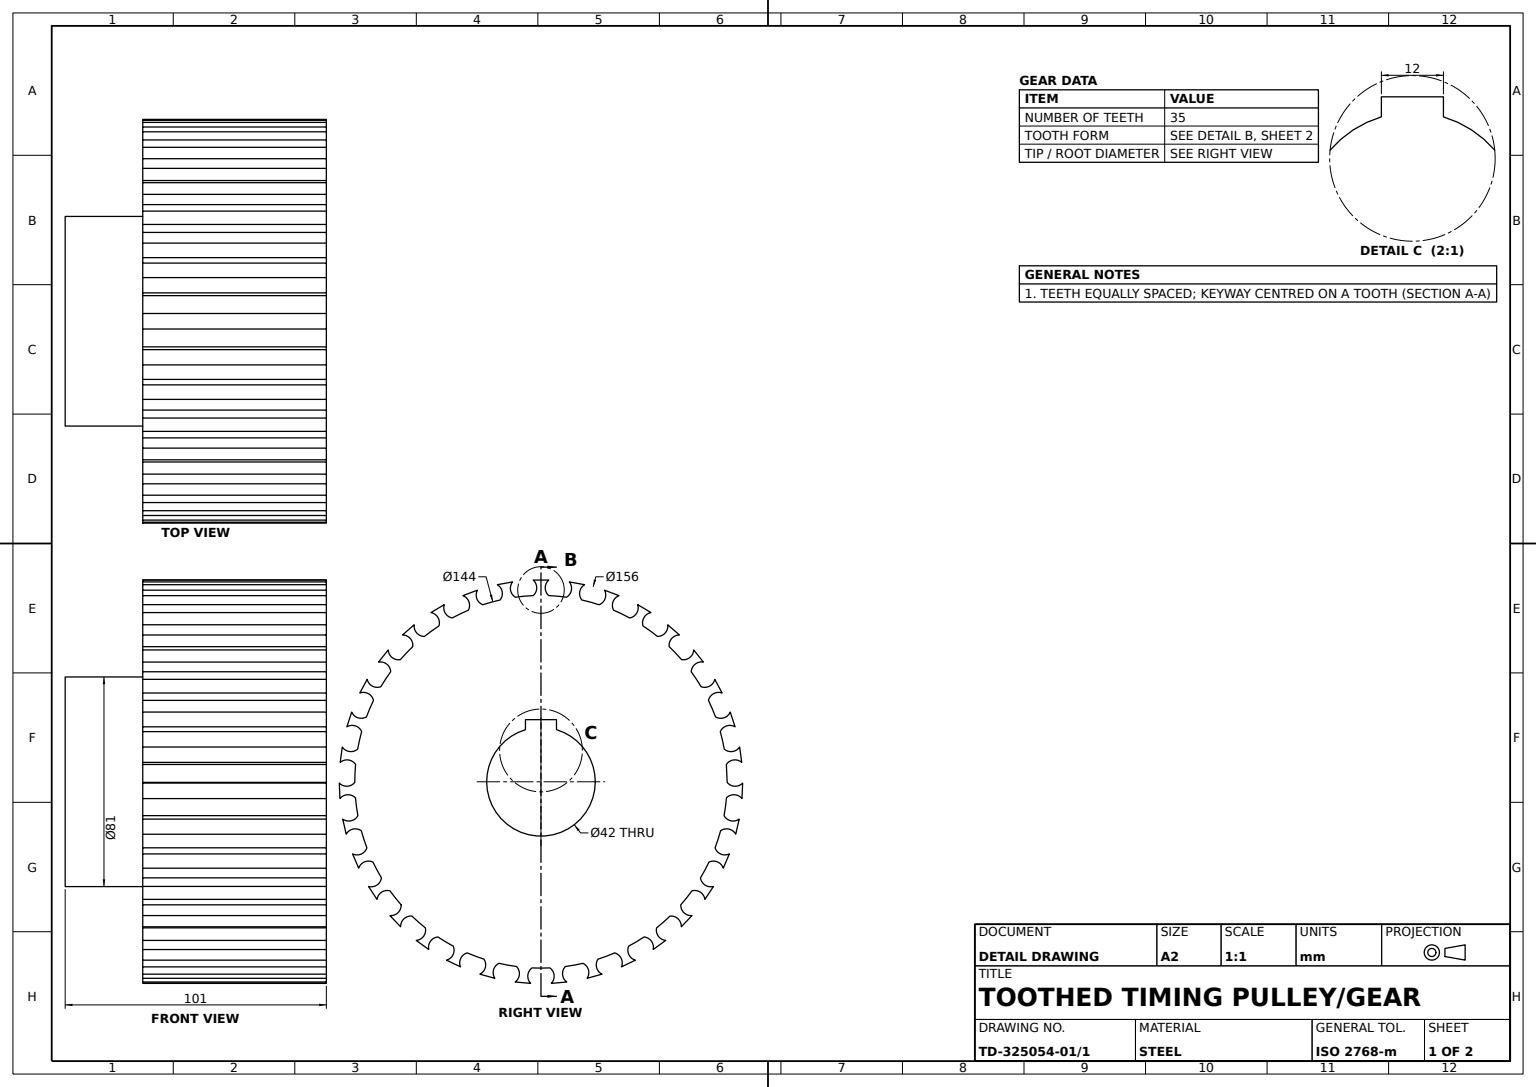
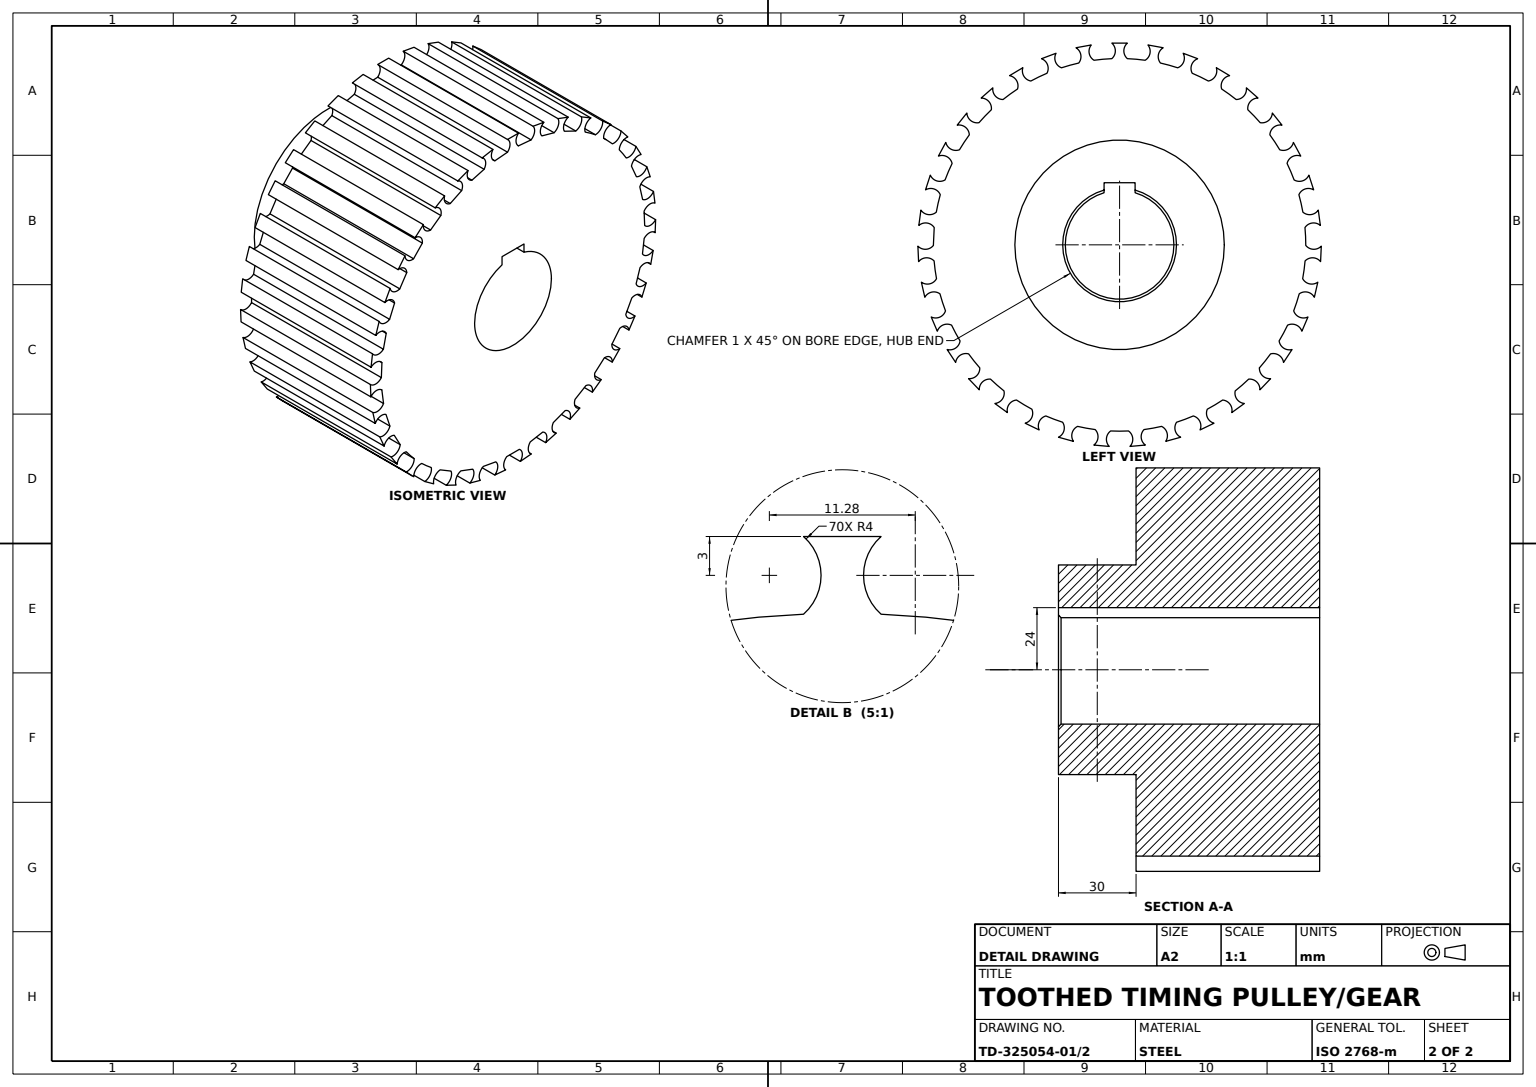
from build123d import *

# Parameters (mm, degrees)
GEAR_BODY_35T_DEPTH       = 71
HUB_SKETCH_R              = 40.5
HUB_81_DEPTH              = 30
BORE_42_WITH_KEYWAY_DEPTH = 150.561858306
EDGE_CHAMFER_1X45_SIZE    = 1


with BuildPart() as part:
    # Gear Tooth Profile Sketch → Gear Body 35T (new body)
    with BuildSketch(Plane.XY):
        with BuildLine():
            ThreePointArc((2.999348888, 77.942311399), (0, 78), (-2.999348888, 77.942311399))
            ThreePointArc((-2.999348888, 77.942311399), (-1.642369889, 74.9399057), (-2.999348888, 71.9375))
            ThreePointArc((-2.999348888, 71.9375), (-6.454030241, 71.710149168), (-9.893788502, 71.316989204))
            ThreePointArc((-9.893788502, 71.316989204), (-11.765060529, 74.028847052), (-10.96598898, 77.225300813))
            ThreePointArc((-10.96598898, 77.225300813), (-13.927437794, 76.746507911), (-16.868285214, 76.154191966))
            ThreePointArc((-16.868285214, 76.154191966), (-14.997013188, 73.442334117), (-15.796084737, 70.245880356))
            ThreePointArc((-15.796084737, 70.245880356), (-19.154652881, 69.40532597), (-22.468931389, 68.404291694))
            ThreePointArc((-22.468931389, 68.404291694), (-24.794352221, 70.738440349), (-24.578870939, 74.026205518))
            ThreePointArc((-24.578870939, 74.026205518), (-27.407236278, 73.02631991), (-30.195060974, 71.918414142))
            ThreePointArc((-30.195060974, 71.918414142), (-27.869640143, 69.584265487), (-28.085121425, 66.296500319))
            ThreePointArc((-28.085121425, 66.296500319), (-31.239629216, 64.869758489), (-34.321904334, 63.293023967))
            ThreePointArc((-34.321904334, 63.293023967), (-37.026733032, 65.17444197), (-37.401767762, 68.447847068))
            ThreePointArc((-37.401767762, 68.447847068), (-40.006143638, 66.959005901), (-42.55134263, 65.371119314))
            ThreePointArc((-42.55134263, 65.371119314), (-39.846513932, 63.489701311), (-39.471479203, 60.216296213))
            ThreePointArc((-39.471479203, 60.216296213), (-42.320538165, 58.249223595), (-45.071743033, 56.147466371))
            ThreePointArc((-45.071743033, 56.147466371), (-48.069044178, 57.5156834), (-49.022540995, 60.669518495))
            ThreePointArc((-49.022540995, 60.669518495), (-51.319220623, 58.739574348), (-53.539989123, 56.722742923))
            ThreePointArc((-53.539989123, 56.722742923), (-50.542687978, 55.354525895), (-49.589191161, 52.2006908))
            ThreePointArc((-49.589191161, 52.2006908), (-52.041230196, 49.756510727), (-54.372938826, 47.197283009))
            ThreePointArc((-54.372938826, 47.197283009), (-57.566376692, 48.008323441), (-59.067689425, 50.941221678))
            ThreePointArc((-59.067689425, 50.941221678), (-60.982855633, 48.632204545), (-62.807816312, 46.251250903))
            ThreePointArc((-62.807816312, 46.251250903), (-59.614378446, 45.440210471), (-58.113065714, 42.507312234))
            ThreePointArc((-58.113065714, 42.507312234), (-60.089274268, 39.664582665), (-61.926543627, 36.730140136))
            ThreePointArc((-61.926543627, 36.730140136), (-65.213478494, 36.957936466), (-67.214353715, 39.575632082))
            ThreePointArc((-67.214353715, 39.575632082), (-68.686451485, 36.961755673), (-70.056948606, 34.293205624))
            ThreePointArc((-70.056948606, 34.293205624), (-66.77001374, 34.065409294), (-64.769138519, 31.447713678))
            ThreePointArc((-64.769138519, 31.447713678), (-66.205999624, 28.297802279), (-67.489778363, 25.082460337))
            ThreePointArc((-67.489778363, 25.082460337), (-70.764565439, 24.719691003), (-73.200693373, 26.938049107))
            ThreePointArc((-73.200693373, 26.938049107), (-74.182408271, 24.103325561), (-75.05439293, 21.232948499))
            ThreePointArc((-75.05439293, 21.232948499), (-71.779605853, 21.595717833), (-69.343477919, 19.377359729))
            ThreePointArc((-69.343477919, 19.377359729), (-70.194809677, 16.021507245), (-70.883836091, 12.628609625))
            ThreePointArc((-70.883836091, 12.628609625), (-74.041221026, 11.686934333), (-76.834302516, 13.43465507))
            ThreePointArc((-76.834302516, 13.43465507), (-77.294081418, 10.470194734), (-77.639527309, 7.490246939))
            ThreePointArc((-77.639527309, 7.490246939), (-74.482142374, 8.431922232), (-71.689060884, 6.684201494))
            ThreePointArc((-71.689060884, 6.684201494), (-71.927500791, 3.230267785), (-71.999629003, -0.23113499))
            ThreePointArc((-71.999629003, -0.23113499), (-74.938130848, -1.721450024), (-77.998393957, -0.500539835))
            ThreePointArc((-77.998393957, -0.500539835), (-77.92145919, -3.499456767), (-77.729263399, -6.493197321))
            ThreePointArc((-77.729263399, -6.493197321), (-74.790761555, -5.002882288), (-71.730498445, -6.223792476))
            ThreePointArc((-71.730498445, -6.223792476), (-71.348382847, -9.664795139), (-70.801294598, -13.083450738))
            ThreePointArc((-70.801294598, -13.083450738), (-73.426467484, -15.07450556), (-76.655552839, -14.419646978))
            ThreePointArc((-76.655552839, -14.419646978), (-76.04437715, -17.356632849), (-75.320717007, -20.267944876))
            ThreePointArc((-75.320717007, -20.267944876), (-72.695544121, -18.276890054), (-69.466458767, -18.931748635))
            ThreePointArc((-69.466458767, -18.931748635), (-68.476069173, -22.249223595), (-67.327348329, -25.515253613))
            ThreePointArc((-67.327348329, -25.515253613), (-69.554817041, -27.943054084), (-72.84893918, -27.875294803))
            ThreePointArc((-72.84893918, -27.875294803), (-71.723166259, -30.655952469), (-70.491300797, -33.391264007))
            ThreePointArc((-70.491300797, -33.391264007), (-68.263832085, -30.963463536), (-64.969709946, -31.031222816))
            ThreePointArc((-64.969709946, -31.031222816), (-63.402878294, -34.118543698), (-61.689445688, -37.126975243))
            ThreePointArc((-61.689445688, -37.126975243), (-63.447617548, -39.913489858), (-66.700900676, -40.435007717))
            ThreePointArc((-66.700900676, -40.435007717), (-65.09671379, -42.969964553), (-63.396236178, -45.441360437))
            ThreePointArc((-63.396236178, -45.441360437), (-61.638064319, -42.654845823), (-58.384781191, -42.133327963))
            ThreePointArc((-58.384781191, -42.133327963), (-56.291866738, -44.891265734), (-54.068793504, -47.545405341))
            ThreePointArc((-54.068793504, -47.545405341), (-55.301159422, -50.601073227), (-58.409040342, -51.695106213))
            ThreePointArc((-58.409040342, -51.695106213), (-56.377999379, -53.902886621), (-54.263564367, -56.030934155))
            ThreePointArc((-54.263564367, -56.030934155), (-53.031198449, -52.975266268), (-49.923317529, -51.881233282))
            ThreePointArc((-49.923317529, -51.881233282), (-47.371588268, -54.221145552), (-44.710325809, -56.43568699))
            ThreePointArc((-44.710325809, -56.43568699), (-45.37727653, -59.662296468), (-48.239865392, -61.29368146))
            ThreePointArc((-48.239865392, -61.29368146), (-45.847249679, -63.103325561), (-43.386816948, -64.819627545))
            ThreePointArc((-43.386816948, -64.819627545), (-42.719866227, -61.593018068), (-39.857277365, -59.961633076))
            ThreePointArc((-39.857277365, -59.961633076), (-36.928747973, -61.808313139), (-33.914831455, -63.512079224))
            ThreePointArc((-33.914831455, -63.512079224), (-33.994930634, -66.80592441), (-36.520221477, -68.922227353))
            ThreePointArc((-36.520221477, -68.922227353), (-33.842931651, -70.275571696), (-31.115581534, -71.524964773))
            ThreePointArc((-31.115581534, -71.524964773), (-31.035482354, -68.231119587), (-28.510191511, -66.114816645))
            ThreePointArc((-28.510191511, -66.114816645), (-25.298987334, -67.408910686), (-22.029286512, -68.547140974))
            ThreePointArc((-22.029286512, -68.547140974), (-21.519959696, -71.802354974), (-23.626787595, -74.335556149))
            ThreePointArc((-23.626787595, -74.335556149), (-20.750873954, -75.189103134), (-17.844265727, -75.931430782))
            ThreePointArc((-17.844265727, -75.931430782), (-18.353592543, -72.676216783), (-16.246764644, -70.143015608))
            ThreePointArc((-16.246764644, -70.143015608), (-12.856096426, -70.842930379), (-9.435702175, -71.379041213))
            ThreePointArc((-9.435702175, -71.379041213), (-8.353319547, -74.490998769), (-9.973969319, -77.359679007))
            ThreePointArc((-9.973969319, -77.359679007), (-6.991866094, -77.685994932), (-3.999420537, -77.89739813))
            ThreePointArc((-3.999420537, -77.89739813), (-5.081803165, -74.785440573), (-3.461153393, -71.916760336))
            ThreePointArc((-3.461153393, -71.916760336), (0, -72), (3.461153393, -71.916760336))
            ThreePointArc((3.461153393, -71.916760336), (5.081803165, -74.785440573), (3.999420537, -77.89739813))
            ThreePointArc((3.999420537, -77.89739813), (6.991866094, -77.685994932), (9.973969319, -77.359679007))
            ThreePointArc((9.973969319, -77.359679007), (8.353319547, -74.490998769), (9.435702175, -71.379041213))
            ThreePointArc((9.435702175, -71.379041213), (12.856096426, -70.842930379), (16.246764644, -70.143015608))
            ThreePointArc((16.246764644, -70.143015608), (18.353592543, -72.676216783), (17.844265727, -75.931430782))
            ThreePointArc((17.844265727, -75.931430782), (20.750873954, -75.189103134), (23.626787595, -74.335556149))
            ThreePointArc((23.626787595, -74.335556149), (21.519959696, -71.802354974), (22.029286512, -68.547140974))
            ThreePointArc((22.029286512, -68.547140974), (25.298987334, -67.408910686), (28.510191511, -66.114816645))
            ThreePointArc((28.510191511, -66.114816645), (31.035482354, -68.231119587), (31.115581534, -71.524964773))
            ThreePointArc((31.115581534, -71.524964773), (33.842931651, -70.275571696), (36.520221477, -68.922227353))
            ThreePointArc((36.520221477, -68.922227353), (33.994930634, -66.80592441), (33.914831455, -63.512079224))
            ThreePointArc((33.914831455, -63.512079224), (36.928747973, -61.808313139), (39.857277365, -59.961633076))
            ThreePointArc((39.857277365, -59.961633076), (42.719866227, -61.593018068), (43.386816948, -64.819627545))
            ThreePointArc((43.386816948, -64.819627545), (45.847249679, -63.103325561), (48.239865392, -61.29368146))
            ThreePointArc((48.239865392, -61.29368146), (45.37727653, -59.662296468), (44.710325809, -56.43568699))
            ThreePointArc((44.710325809, -56.43568699), (47.371588268, -54.221145552), (49.923317529, -51.881233282))
            ThreePointArc((49.923317529, -51.881233282), (53.031198449, -52.975266268), (54.263564367, -56.030934155))
            ThreePointArc((54.263564367, -56.030934155), (56.377999379, -53.902886621), (58.409040342, -51.695106213))
            ThreePointArc((58.409040342, -51.695106213), (55.301159422, -50.601073227), (54.068793504, -47.545405341))
            ThreePointArc((54.068793504, -47.545405341), (56.291866738, -44.891265734), (58.384781191, -42.133327963))
            ThreePointArc((58.384781191, -42.133327963), (61.638064319, -42.654845823), (63.396236178, -45.441360437))
            ThreePointArc((63.396236178, -45.441360437), (65.09671379, -42.969964553), (66.700900676, -40.435007717))
            ThreePointArc((66.700900676, -40.435007717), (63.447617548, -39.913489858), (61.689445688, -37.126975243))
            ThreePointArc((61.689445688, -37.126975243), (63.402878294, -34.118543698), (64.969709946, -31.031222816))
            ThreePointArc((64.969709946, -31.031222816), (68.263832085, -30.963463536), (70.491300797, -33.391264007))
            ThreePointArc((70.491300797, -33.391264007), (71.723166259, -30.655952469), (72.84893918, -27.875294803))
            ThreePointArc((72.84893918, -27.875294803), (69.554817041, -27.943054084), (67.327348329, -25.515253613))
            ThreePointArc((67.327348329, -25.515253613), (68.476069173, -22.249223595), (69.466458767, -18.931748635))
            ThreePointArc((69.466458767, -18.931748635), (72.695544121, -18.276890054), (75.320717007, -20.267944876))
            ThreePointArc((75.320717007, -20.267944876), (76.04437715, -17.356632849), (76.655552839, -14.419646978))
            ThreePointArc((76.655552839, -14.419646978), (73.426467484, -15.07450556), (70.801294598, -13.083450738))
            ThreePointArc((70.801294598, -13.083450738), (71.348382847, -9.664795139), (71.730498445, -6.223792476))
            ThreePointArc((71.730498445, -6.223792476), (74.790761555, -5.002882288), (77.729263399, -6.493197321))
            ThreePointArc((77.729263399, -6.493197321), (77.92145919, -3.499456767), (77.998393957, -0.500539835))
            ThreePointArc((77.998393957, -0.500539835), (74.938130848, -1.721450024), (71.999629003, -0.23113499))
            ThreePointArc((71.999629003, -0.23113499), (71.927500791, 3.230267785), (71.689060884, 6.684201494))
            ThreePointArc((71.689060884, 6.684201494), (74.482142374, 8.431922232), (77.639527309, 7.490246939))
            ThreePointArc((77.639527309, 7.490246939), (77.294081418, 10.470194734), (76.834302516, 13.43465507))
            ThreePointArc((76.834302516, 13.43465507), (74.041221026, 11.686934333), (70.883836091, 12.628609625))
            ThreePointArc((70.883836091, 12.628609625), (70.194809677, 16.021507245), (69.343477919, 19.377359729))
            ThreePointArc((69.343477919, 19.377359729), (71.779605853, 21.595717833), (75.05439293, 21.232948499))
            ThreePointArc((75.05439293, 21.232948499), (74.182408271, 24.103325561), (73.200693373, 26.938049107))
            ThreePointArc((73.200693373, 26.938049107), (70.764565439, 24.719691003), (67.489778363, 25.082460337))
            ThreePointArc((67.489778363, 25.082460337), (66.205999624, 28.297802279), (64.769138519, 31.447713678))
            ThreePointArc((64.769138519, 31.447713678), (66.77001374, 34.065409294), (70.056948606, 34.293205624))
            ThreePointArc((70.056948606, 34.293205624), (68.686451485, 36.961755673), (67.214353715, 39.575632082))
            ThreePointArc((67.214353715, 39.575632082), (65.213478494, 36.957936466), (61.926543627, 36.730140136))
            ThreePointArc((61.926543627, 36.730140136), (60.089274268, 39.664582665), (58.113065714, 42.507312234))
            ThreePointArc((58.113065714, 42.507312234), (59.614378446, 45.440210471), (62.807816312, 46.251250903))
            ThreePointArc((62.807816312, 46.251250903), (60.982855633, 48.632204545), (59.067689425, 50.941221678))
            ThreePointArc((59.067689425, 50.941221678), (57.566376692, 48.008323441), (54.372938826, 47.197283009))
            ThreePointArc((54.372938826, 47.197283009), (52.041230196, 49.756510727), (49.589191161, 52.2006908))
            ThreePointArc((49.589191161, 52.2006908), (50.542687978, 55.354525895), (53.539989123, 56.722742923))
            ThreePointArc((53.539989123, 56.722742923), (51.319220623, 58.739574348), (49.022540995, 60.669518495))
            ThreePointArc((49.022540995, 60.669518495), (48.069044178, 57.5156834), (45.071743033, 56.147466371))
            ThreePointArc((45.071743033, 56.147466371), (42.320538165, 58.249223595), (39.471479203, 60.216296213))
            ThreePointArc((39.471479203, 60.216296213), (39.846513932, 63.489701311), (42.55134263, 65.371119314))
            ThreePointArc((42.55134263, 65.371119314), (40.006143638, 66.959005901), (37.401767762, 68.447847068))
            ThreePointArc((37.401767762, 68.447847068), (37.026733032, 65.17444197), (34.321904334, 63.293023967))
            ThreePointArc((34.321904334, 63.293023967), (31.239629216, 64.869758489), (28.085121425, 66.296500319))
            ThreePointArc((28.085121425, 66.296500319), (27.869640143, 69.584265487), (30.195060974, 71.918414142))
            ThreePointArc((30.195060974, 71.918414142), (27.407236278, 73.02631991), (24.578870939, 74.026205518))
            ThreePointArc((24.578870939, 74.026205518), (24.794352221, 70.738440349), (22.468931389, 68.404291694))
            ThreePointArc((22.468931389, 68.404291694), (19.154652881, 69.40532597), (15.796084737, 70.245880356))
            ThreePointArc((15.796084737, 70.245880356), (14.997013188, 73.442334117), (16.868285214, 76.154191966))
            ThreePointArc((16.868285214, 76.154191966), (13.927437794, 76.746507911), (10.96598898, 77.225300813))
            ThreePointArc((10.96598898, 77.225300813), (11.765060529, 74.028847052), (9.893788502, 71.316989204))
            ThreePointArc((9.893788502, 71.316989204), (6.454030241, 71.710149168), (2.999348888, 71.9375))
            ThreePointArc((2.999348888, 71.9375), (1.642369889, 74.9399057), (2.999348888, 77.942311399))
        make_face()
    extrude(amount=GEAR_BODY_35T_DEPTH)

    # Hub Sketch → Hub Ø81 (add)
    with BuildSketch(Plane.XY.offset(71)):
        with Locations(Location((0, 0, 0), (0, 0, 180))):
            Circle(HUB_SKETCH_R)
    extrude(amount=HUB_81_DEPTH)

    # Bore Keyway Sketch → Bore Ø42 with Keyway (cut, through all)
    with BuildSketch(Plane.XY.offset(101)):
        with BuildLine():
            Line((-6, 24), (6, 24))
            Line((6, 24), (6, 20.124611797))
            ThreePointArc((6, 20.124611797), (0, -21), (-6, 20.124611797))
            Line((-6, 20.124611797), (-6, 24))
        make_face()
    extrude(amount=-BORE_42_WITH_KEYWAY_DEPTH, mode=Mode.SUBTRACT)

    # Edge Chamfer 1x45
    edge_chamfer_1x45_edges = [part.edges().sort_by_distance(p)[0] for p in [
        (0, -21, 101),
    ]]
    chamfer(edge_chamfer_1x45_edges, length=EDGE_CHAMFER_1X45_SIZE)


solid = part.part
